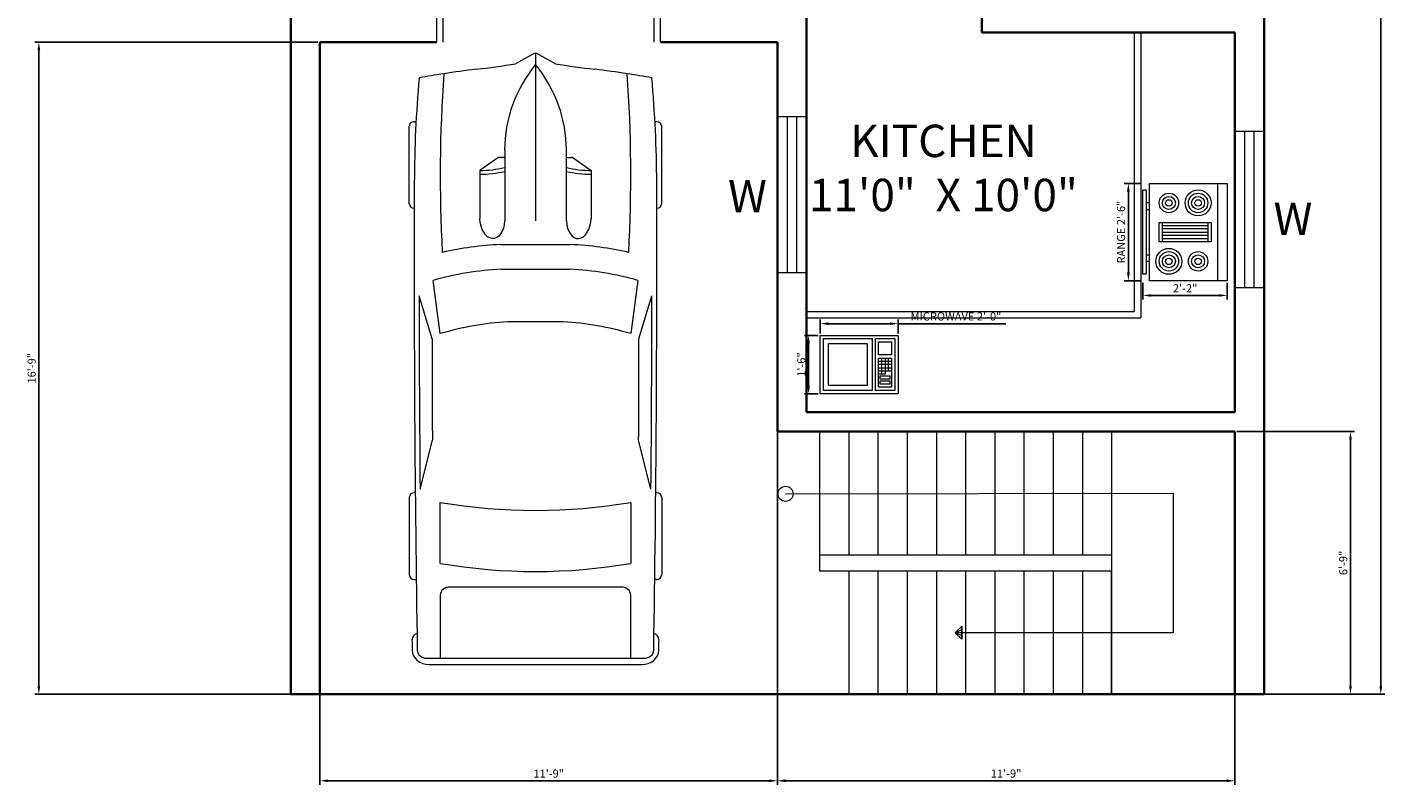
# Model space of a CAD drawing. Units: inches. Extents: x 2318 to 3542, y 1525 to 2117.
# Tile 1 of 6: x 2320 to 2739, y 1525 to 1758. Entities that reach past the tile are written whole.
import ezdxf

# ---------------------------------------------------------------- set-up
doc = ezdxf.new("R2010")
doc.units = ezdxf.units.IN
for name, color, linetype, lineweight in [('A-ANNO-DIMS', 2, 'Continuous', 18), ('A-ANNO-SYMB', 2, 'Continuous', 13), ('A-ANNO-TEXT', 7, 'Continuous', 18), ('A-AREA-IDEN', 7, 'Continuous', 25), ('A-DOOR', 4, 'Continuous', 18), ('A-EQPM', 9, 'Continuous', 18), ('A-FLOR-CASE', 8, 'Continuous', 18), ('A-FLOR-STRS', 3, 'Continuous', 18), ('A-GLAZ', 4, 'Continuous', 18), ('A-WALL', 7, 'Continuous', 35), ('C-PRKG', 8, 'Continuous', 13)]:
    doc.layers.add(name, color=color, linetype=linetype, lineweight=lineweight)
doc.styles.add('Annotative', font='arial.ttf')
doc.styles.get("Standard").update_dxf_attribs({"font": 'arial.ttf'})
doc.dimstyles.new('ISO-25', dxfattribs={"dimtxt": 2.5, "dimasz": 2.5, "dimexe": 1.25, "dimexo": 0.625, "dimtad": 1, "dimdec": 0, "dimlunit": 3, "dimtxsty": 'Standard', "dimcen": 2.5, "dimadec": 0, "dimazin": 0, "dimtfac": 1, "dimtdec": 0, "dimtmove": 0, "dimatfit": 3, "dimfxl": 1, "dimarcsym": 0})

# ---------------------------------------------------------------- blocks, each defined once
blk = doc.blocks.new('Range-Oven - 30 in top')
for p, q in [((0, -3), (30, -3)), ((12, -6), (18, -6)), ((13, -20), (13, -6)), ((14, -6), (14, -20)), ((15, -20), (15, -6)), ((16, -6), (16, -20)), ((17, -20), (17, -6)), ((18, -20), (12, -20)), ((6, -24), (6, -25)), ((8, -25), (8, -24)), ((22, -25), (22, -24)), ((24, -24), (24, -25))]:
    blk.add_line(p, q)
for points in [[(0, -24), (0, 0), (30, 0), (30, -24)], [(12, -21), (12, -5), (18, -5), (18, -21)], [(2, -26), (2, -25), (28, -25), (28, -26)]]:
    blk.add_lwpolyline(points, close=True)
for centre, radius in [((6, -9), 4), ((6, -9), 3), ((6, -9), 2), ((6, -9), 1), ((24, -9), 3), ((24, -9), 2), ((24, -9), 1), ((6, -18), 3), ((6, -18), 2), ((24, -18), 4), ((24, -18), 3), ((24, -18), 2), ((6, -18), 1), ((24, -18), 1)]:
    blk.add_circle(centre, radius)
blk = doc.blocks.new('Microwave')
for p, q in [((18, 10), (22, 10)), ((22, 9), (18, 9)), ((19, 7), (19, 11)), ((20, 11), (20, 7)), ((21, 7), (21, 11)), ((18, 8), (22, 8)), ((22, 7), (18, 7)), ((20, 6), (18, 6)), ((19, 6), (19, 7)), ((20, 7), (20, 6))]:
    blk.add_line(p, q)
for points in [[(0, 0), (0, 18), (24, 18), (24, 0)], [(1, 1), (1, 17), (16, 17), (16, 1)], [(17, 1), (17, 17), (23, 17), (23, 1)], [(2.5, 2.5), (2.5, 15.5), (14.5, 15.5), (14.5, 2.5)], [(18, 12), (18, 16), (22, 16), (22, 12)], [(18, 2), (18, 11), (22, 11), (22, 2)], [(18.5, 4.5), (18.5, 5.5), (21.5, 5.5), (21.5, 4.5)], [(18.5, 3), (18.5, 4), (21.5, 4), (21.5, 3)]]:
    blk.add_lwpolyline(points, close=True)
blk = doc.blocks.new('*U12')
for p, q in [((1182, 988), (568, 988)), ((3472, 988), (4087, 988)), ((536, 950), (536, 936)), ((1214, 950), (1214, 950)), ((2235, 810), (1899, 912)), ((3412, 904), (3030, 807)), ((3440, 942), (3440, 950)), ((4119, 950), (4119, 934)), ((4736, -851), (4736, 851)), ((1779, 801), (2195, 746)), ((3516, 746), (3994, 746)), ((4736, 746), (4242, 746)), ((4785, -832), (4785, 832)), ((4179, 670), (4179, -670)), ((820, 295), (918, 436)), ((918, 436), (1294, 436)), ((756, 241), (1313, 241)), ((816, 241), (816, 283)), ((1496, -274), (1496, 274)), ((1690, -267), (1690, 267)), ((2102, 216), (2102, -216)), ((4736, -267), (4736, 267)), ((83, 156), (3, 10)), ((0, 0), (1313, 0)), ((3, -10), (83, -156)), ((756, -241), (1313, -241)), ((816, -241), (816, -283)), ((820, -295), (918, -436)), ((918, -436), (1294, -436)), ((2195, -746), (1779, -801)), ((2235, -810), (1899, -912)), ((3412, -904), (3030, -807)), ((3994, -746), (3516, -746)), ((4242, -746), (4736, -746)), ((536, -950), (536, -936)), ((1214, -950), (1214, -950)), ((3440, -942), (3440, -950)), ((4119, -950), (4119, -934)), ((1182, -988), (568, -988)), ((3472, -988), (4087, -988))]:
    blk.add_line(p, q)
for centre, major_axis, ratio, start_param, end_param in [((568, 950), (0, -37.6), 0.842304, 3.141593, 4.712389), ((1182, 950), (0, 37.6), 0.842304, -1.570796, 0), ((3472, 950), (0, -37.6), 0.842304, 3.141593, 4.712389), ((4087, 950), (0, 37.6), 0.842304, -1.570796, 0), ((4588, 910), (0, 56.4), 0.842304, -0.013017, 1.249894), ((1638, -268131), (0, 269121), 0.842304, -0.013397, -0.013017), ((4673, 832), (0, -133), 0.842304, 1.570796, 3.128196), ((6757, -699), (0, 7958), 0.842304, 1.367076, 1.39176), ((1046, -12468), (0, 13417), 0.842304, 0.00281, 0.075598), ((1638, -268113), (0, 269063), 0.842304, -0.013397, 0.002797), ((1638, -268113), (0, -269025), 0.842304, 3.133765, 3.140441), ((4673, 851), (0, -75.2), 0.842304, 1.570796, 3.128196), ((952, -15087), (0, -15833), 0.842304, 3.096046, 3.200911), ((3436, 137), (0, 2077), 0.842304, 1.245306, 1.50788), ((3800, 71), (0, -2021), 0.842304, 4.372215, 4.640744), ((2433, -93125), (0, -93935), 0.842304, 3.134049, 3.144098), ((434, 0), (0, 3734), 0.842304, 4.511394, 4.913384), ((912, 0), (0, 3734), 0.842304, 4.511394, 4.913384), ((4242, 670), (0, 75.2), 0.842304, 0, 1.570796), ((6583, -699), (0, -7755), 0.842304, 4.528606, 4.561838), ((3414, 137), (0, -2280), 0.842304, 4.449482, 4.652344), ((-5194, 1331), (0, -6374), 0.842304, 1.385369, 1.434372), ((331, 432), (0, 696), 0.842304, 4.435146, 4.718221), ((361, 432), (0, 696), 0.842304, 4.435146, 4.718221), ((1290, 339), (161, -9), 0.603834, -1.395552, 1.581315), ((756, -1185), (0, 1427), 0.842304, 0, 0.590319), ((832, 283), (0, 18.8), 0.842304, 0.879714, 1.570796), ((16, 0), (0, -18.8), 0.842304, 4.131459, 5.293319), ((756, 1185), (0, 1427), 0.842304, 2.551274, 3.141593), ((-5194, -1331), (0, 6374), 0.842304, -1.434372, -1.385369), ((832, -283), (0, -18.8), 0.842304, 4.712389, 5.403472), ((331, -432), (0, -696), 0.842304, 1.564964, 1.848039), ((361, -432), (0, -696), 0.842304, 1.564964, 1.848039), ((3414, -137), (0, -2280), 0.842304, -1.510751, -1.307889), ((3436, -137), (0, -2077), 0.842304, -1.50788, -1.245306), ((3800, -71), (0, -2021), 0.842304, -1.499151, -1.230623), ((6583, 699), (0, 7755), 0.842304, 1.721348, 1.754579), ((6757, 699), (0, 7958), 0.842304, 1.749832, 1.774517), ((952, 15087), (0, -15833), 0.842304, -0.059319, 0.045547), ((4242, -670), (0, -75.2), 0.842304, 4.712389, 6.283185), ((2433, 93125), (0, -93935), 0.842304, -0.002505, 0.007544), ((4673, -832), (0, -133), 0.842304, 0.013397, 1.570796), ((1046, 12468), (0, -13417), 0.842304, -0.075598, -0.00281), ((568, -950), (0, 37.6), 0.842304, 1.570796, 3.141593), ((1638, 268113), (0, 269063), 0.842304, 3.138796, 3.15499), ((1182, -950), (0, -37.6), 0.842304, 0, 1.570796), ((1638, 268113), (0, -269025), 0.842304, 0.001152, 0.007828), ((3472, -950), (0, -37.6), 0.842304, -1.570796, 0), ((4087, -950), (0, 37.6), 0.842304, 3.141593, 4.712389), ((4588, -910), (0, -56.4), 0.842304, -1.249894, 0.013017), ((4673, -851), (0, 75.2), 0.842304, 3.15499, 4.712389), ((1638, 268131), (0, 269121), 0.842304, 3.15461, 3.15499)]:
    blk.add_ellipse(centre, major_axis=major_axis, ratio=ratio, start_param=start_param, end_param=end_param)
at = {"extrusion": (0, 0, -1)}
blk.add_ellipse((1290, -339), major_axis=(161, 9), ratio=0.603834, start_param=-1.395552, end_param=1.581315, dxfattribs=at)
blk = doc.blocks.new('*D16')
at = {"layer": 'A-ANNO-DIMS', "color": 0, "lineweight": -2, "transparency": 16777216}
for p, q in [((2702.28, 2032.62), (2738.91, 2032.62)), ((2737.66, 1555.12), (2737.66, 2030.12)), ((2702.28, 1552.62), (2738.91, 1552.62))]:
    blk.add_line(p, q, dxfattribs=at)
at = {"layer": 'A-ANNO-DIMS', "color": 0, "transparency": 16777216}
for points in [[(2737.24, 2030.12), (2738.07, 2030.12), (2737.66, 2032.62)], [(2737.24, 1555.12), (2738.07, 1555.12), (2737.66, 1552.62)]]:
    blk.add_solid(points, dxfattribs=at)
at = {"layer": 'Defpoints', "color": 0, "transparency": 16777216}
for p in [(2701.66, 2032.62), (2737.66, 2032.62), (2701.66, 1552.62)]:
    blk.add_point(p, dxfattribs=at)
at = {"layer": 'A-ANNO-DIMS', "color": 0, "transparency": 16777216, "insert": (2735.76, 1792.62), "char_height": 2.5, "attachment_point": 5, "rotation": 90}
blk.add_mtext("40'", dxfattribs=at)
blk = doc.blocks.new('WIN-48x9')
for p, q in [((48, 9), (0, 9)), ((0, 9), (0, 0)), ((48, 0), (48, 9)), ((48, 6), (0, 6)), ((0, 3), (48, 3)), ((0, 0), (48, 0))]:
    blk.add_line(p, q)
blk = doc.blocks.new('STAIR-ARROWHEAD')
for p, q in [((0, 2), (2, 4)), ((0, 2), (2, 3)), ((2, 2), (0, 2)), ((2, 0), (0, 2)), ((2, 1), (0, 2)), ((2, 2), (2, 4)), ((2, 4), (2, 2)), ((2, 4), (2, 0)), ((2, 3), (2, 1)), ((2, 2), (2, 0)), ((2, 0), (2, 2))]:
    blk.add_line(p, q)
blk = doc.blocks.new('*D46')
at = {"layer": 'A-ANNO-DIMS', "color": 0, "lineweight": -2, "transparency": 16777216}
for p, q in [((2663.72, 1710.07), (2658.59, 1710.07)), ((2659.84, 1707.57), (2659.84, 1682.57)), ((2663.72, 1680.07), (2658.59, 1680.07))]:
    blk.add_line(p, q, dxfattribs=at)
at = {"layer": 'A-ANNO-DIMS', "color": 0, "transparency": 16777216}
for points in [[(2659.42, 1707.57), (2660.26, 1707.57), (2659.84, 1710.07)], [(2659.42, 1682.57), (2660.26, 1682.57), (2659.84, 1680.07)]]:
    blk.add_solid(points, dxfattribs=at)
at = {"layer": 'Defpoints', "color": 0, "transparency": 16777216}
for p in [(2664.34, 1710.07), (2659.84, 1680.07), (2664.34, 1680.07)]:
    blk.add_point(p, dxfattribs=at)
at = {"layer": 'A-ANNO-DIMS', "color": 0, "transparency": 16777216, "insert": (2657.92, 1695.07), "char_height": 2.5, "attachment_point": 5, "rotation": 90}
blk.add_mtext('RANGE 2\'-6"', dxfattribs=at)
blk = doc.blocks.new('*D47')
at = {"layer": 'A-ANNO-DIMS', "color": 0, "lineweight": -2, "transparency": 16777216}
for p, q in [((2664.34, 1679.44), (2664.34, 1674.32)), ((2690.34, 1679.44), (2690.34, 1674.32)), ((2666.84, 1675.57), (2687.84, 1675.57))]:
    blk.add_line(p, q, dxfattribs=at)
at = {"layer": 'A-ANNO-DIMS', "color": 0, "transparency": 16777216}
for points in [[(2666.84, 1675.98), (2666.84, 1675.15), (2664.34, 1675.57)], [(2687.84, 1675.98), (2687.84, 1675.15), (2690.34, 1675.57)]]:
    blk.add_solid(points, dxfattribs=at)
at = {"layer": 'Defpoints', "color": 0, "transparency": 16777216}
for p in [(2664.34, 1680.07), (2690.34, 1680.07), (2690.34, 1675.57)]:
    blk.add_point(p, dxfattribs=at)
at = {"layer": 'A-ANNO-DIMS', "color": 0, "transparency": 16777216, "insert": (2677.34, 1677.45), "char_height": 2.5, "attachment_point": 5}
blk.add_mtext('2\'-2"', dxfattribs=at)
blk = doc.blocks.new('*D48')
at = {"layer": 'A-ANNO-DIMS', "color": 0, "lineweight": -2, "transparency": 16777216}
for p, q in [((2564.87, 1663.88), (2564.87, 1668.11)), ((2567.37, 1666.86), (2586.37, 1666.86)), ((2588.87, 1663.88), (2588.87, 1668.11)), ((2588.87, 1666.86), (2622.04, 1666.86))]:
    blk.add_line(p, q, dxfattribs=at)
at = {"layer": 'A-ANNO-DIMS', "color": 0, "transparency": 16777216}
for points in [[(2567.37, 1667.27), (2567.37, 1666.44), (2564.87, 1666.86)], [(2586.37, 1667.27), (2586.37, 1666.44), (2588.87, 1666.86)]]:
    blk.add_solid(points, dxfattribs=at)
at = {"layer": 'Defpoints', "color": 0, "transparency": 16777216}
for p in [(2588.87, 1666.86), (2564.87, 1663.26), (2588.87, 1663.26)]:
    blk.add_point(p, dxfattribs=at)
at = {"layer": 'A-ANNO-DIMS', "color": 0, "transparency": 16777216, "insert": (2606.7, 1668.77), "char_height": 2.5, "attachment_point": 5}
blk.add_mtext('MICROWAVE 2\'-0"', dxfattribs=at)
blk = doc.blocks.new('*D49')
at = {"layer": 'A-ANNO-DIMS', "color": 0, "lineweight": -2, "transparency": 16777216}
for p, q in [((2564.24, 1663.26), (2560.02, 1663.26)), ((2561.27, 1647.76), (2561.27, 1660.76)), ((2564.24, 1645.26), (2560.02, 1645.26))]:
    blk.add_line(p, q, dxfattribs=at)
at = {"layer": 'A-ANNO-DIMS', "color": 0, "transparency": 16777216}
for points in [[(2560.85, 1660.76), (2561.68, 1660.76), (2561.27, 1663.26)], [(2560.85, 1647.76), (2561.68, 1647.76), (2561.27, 1645.26)]]:
    blk.add_solid(points, dxfattribs=at)
at = {"layer": 'Defpoints', "color": 0, "transparency": 16777216}
for p in [(2561.27, 1663.26), (2564.87, 1663.26), (2564.87, 1645.26)]:
    blk.add_point(p, dxfattribs=at)
at = {"layer": 'A-ANNO-DIMS', "color": 0, "transparency": 16777216, "insert": (2559.36, 1654.26), "char_height": 2.5, "attachment_point": 5, "rotation": 90}
blk.add_mtext('1\'-6"', dxfattribs=at)
blk = doc.blocks.new('*D51')
at = {"layer": 'A-ANNO-DIMS', "color": 0, "lineweight": -2, "transparency": 16777216}
for p, q in [((2410.66, 1752.99), (2410.66, 1524.72)), ((2551.66, 1752.99), (2551.66, 1524.72)), ((2413.16, 1525.97), (2549.16, 1525.97))]:
    blk.add_line(p, q, dxfattribs=at)
at = {"layer": 'A-ANNO-DIMS', "color": 0, "transparency": 16777216}
for points in [[(2413.16, 1526.39), (2413.16, 1525.55), (2410.66, 1525.97)], [(2549.16, 1526.39), (2549.16, 1525.55), (2551.66, 1525.97)]]:
    blk.add_solid(points, dxfattribs=at)
at = {"layer": 'Defpoints', "color": 0, "transparency": 16777216}
for p in [(2410.66, 1753.62), (2551.66, 1753.62), (2551.66, 1525.97)]:
    blk.add_point(p, dxfattribs=at)
at = {"layer": 'A-ANNO-DIMS', "color": 0, "transparency": 16777216, "insert": (2481.16, 1527.87), "char_height": 2.5, "attachment_point": 5}
blk.add_mtext('11\'-9"', dxfattribs=at)
blk = doc.blocks.new('*D52')
at = {"layer": 'A-ANNO-DIMS', "color": 0, "lineweight": -2, "transparency": 16777216}
for p, q in [((2410.03, 1753.62), (2322.76, 1753.62)), ((2324.01, 1555.12), (2324.01, 1751.12)), ((2410.03, 1552.62), (2322.76, 1552.62))]:
    blk.add_line(p, q, dxfattribs=at)
at = {"layer": 'A-ANNO-DIMS', "color": 0, "transparency": 16777216}
for points in [[(2323.59, 1751.12), (2324.42, 1751.12), (2324.01, 1753.62)], [(2323.59, 1555.12), (2324.42, 1555.12), (2324.01, 1552.62)]]:
    blk.add_solid(points, dxfattribs=at)
at = {"layer": 'Defpoints', "color": 0, "transparency": 16777216}
for p in [(2324.01, 1753.62), (2410.66, 1753.62), (2410.66, 1552.62)]:
    blk.add_point(p, dxfattribs=at)
at = {"layer": 'A-ANNO-DIMS', "color": 0, "transparency": 16777216, "insert": (2322.11, 1653.12), "char_height": 2.5, "attachment_point": 5, "rotation": 90}
blk.add_mtext('16\'-9"', dxfattribs=at)
blk = doc.blocks.new('*D59')
at = {"layer": 'A-ANNO-DIMS', "color": 0, "lineweight": -2, "transparency": 16777216}
for p, q in [((2551.66, 1632.99), (2551.66, 1524.72)), ((2692.66, 1632.99), (2692.66, 1524.72)), ((2554.16, 1525.97), (2690.16, 1525.97))]:
    blk.add_line(p, q, dxfattribs=at)
at = {"layer": 'A-ANNO-DIMS', "color": 0, "transparency": 16777216}
for points in [[(2554.16, 1526.39), (2554.16, 1525.55), (2551.66, 1525.97)], [(2690.16, 1526.39), (2690.16, 1525.55), (2692.66, 1525.97)]]:
    blk.add_solid(points, dxfattribs=at)
at = {"layer": 'Defpoints', "color": 0, "transparency": 16777216}
for p in [(2551.66, 1633.62), (2692.66, 1633.62), (2692.66, 1525.97)]:
    blk.add_point(p, dxfattribs=at)
at = {"layer": 'A-ANNO-DIMS', "color": 0, "transparency": 16777216, "insert": (2622.16, 1527.87), "char_height": 2.5, "attachment_point": 5}
blk.add_mtext('11\'-9"', dxfattribs=at)
blk = doc.blocks.new('*D60')
at = {"layer": 'A-ANNO-DIMS', "color": 0, "lineweight": -2, "transparency": 16777216}
for p, q in [((2693.28, 1633.62), (2729.56, 1633.62)), ((2728.31, 1555.12), (2728.31, 1631.12)), ((2693.28, 1552.62), (2729.56, 1552.62))]:
    blk.add_line(p, q, dxfattribs=at)
at = {"layer": 'A-ANNO-DIMS', "color": 0, "transparency": 16777216}
for points in [[(2727.89, 1631.12), (2728.72, 1631.12), (2728.31, 1633.62)], [(2727.89, 1555.12), (2728.72, 1555.12), (2728.31, 1552.62)]]:
    blk.add_solid(points, dxfattribs=at)
at = {"layer": 'Defpoints', "color": 0, "transparency": 16777216}
for p in [(2692.66, 1633.62), (2728.31, 1633.62), (2692.66, 1552.62)]:
    blk.add_point(p, dxfattribs=at)
at = {"layer": 'A-ANNO-DIMS', "color": 0, "transparency": 16777216, "insert": (2726.41, 1593.12), "char_height": 2.5, "attachment_point": 5, "rotation": 90}
blk.add_mtext('6\'-9"', dxfattribs=at)

msp = doc.modelspace()

# ---------------------------------------------------------------- linework, layer by layer
at = {"layer": 'A-ANNO-SYMB'}
for p, q in [((2554.18, 1614.42), (2673.66, 1614.62)), ((2673.66, 1614.62), (2673.66, 1571.62)), ((2673.66, 1571.62), (2608.49, 1571.62))]:
    msp.add_line(p, q, dxfattribs=at)
msp.add_circle((2554.18, 1614.42), 2.33, dxfattribs=at)
at = {"layer": 'A-DOOR'}
for p, q in [((2446.66, 1753.62), (2446.66, 1762.62)), ((2448.66, 1753.62), (2448.66, 1762.62)), ((2513.66, 1753.62), (2513.66, 1762.62)), ((2515.66, 1753.62), (2515.66, 1762.62))]:
    msp.add_line(p, q, dxfattribs=at)
at = {"layer": 'A-FLOR-CASE'}
for p, q in [((2661.66, 1756.62), (2661.66, 1670.62)), ((2663.66, 1756.62), (2663.66, 1668.62)), ((2560.66, 1670.62), (2661.66, 1670.62)), ((2560.66, 1668.62), (2663.66, 1668.62))]:
    msp.add_line(p, q, dxfattribs=at)
at = {"layer": 'A-FLOR-STRS'}
for p, q in [((2564.66, 1633.62), (2564.66, 1590.62)), ((2573.66, 1633.62), (2573.66, 1595.62)), ((2582.66, 1633.62), (2582.66, 1595.62)), ((2591.66, 1633.62), (2591.66, 1595.62)), ((2600.66, 1633.62), (2600.66, 1595.62)), ((2609.66, 1633.62), (2609.66, 1595.62)), ((2618.66, 1633.62), (2618.66, 1595.62)), ((2627.66, 1633.62), (2627.66, 1595.62)), ((2636.66, 1633.62), (2636.66, 1595.62)), ((2645.66, 1633.62), (2645.66, 1595.62)), ((2654.66, 1633.62), (2654.66, 1595.62)), ((2564.66, 1595.62), (2654.66, 1595.62)), ((2654.66, 1595.62), (2654.66, 1590.62)), ((2654.66, 1590.62), (2564.66, 1590.62)), ((2573.66, 1590.62), (2573.66, 1552.62)), ((2582.66, 1590.62), (2582.66, 1552.62)), ((2591.66, 1590.62), (2591.66, 1552.62)), ((2600.66, 1590.62), (2600.66, 1552.62)), ((2609.66, 1590.62), (2609.66, 1552.62)), ((2618.66, 1590.62), (2618.66, 1552.62)), ((2627.66, 1590.62), (2627.66, 1552.62)), ((2636.66, 1590.62), (2636.66, 1552.62)), ((2645.66, 1590.62), (2645.66, 1552.62)), ((2654.66, 1590.62), (2654.66, 1552.62)), ((2654.66, 1552.62), (2654.66, 1590.62))]:
    msp.add_line(p, q, dxfattribs=at)
at = {"layer": 'A-WALL'}
for p, q in [((2401.66, 1552.62), (2401.66, 2032.62)), ((2701.66, 2032.62), (2701.66, 1552.62)), ((2560.66, 1756.62), (2560.66, 1762.62)), ((2614.66, 1762.62), (2614.66, 1756.62)), ((2410.66, 1552.62), (2410.66, 1753.62)), ((2410.66, 1753.62), (2446.66, 1753.62)), ((2410.66, 1753.62), (2446.66, 1753.62)), ((2551.66, 1753.62), (2515.66, 1753.62)), ((2515.66, 1753.62), (2551.66, 1753.62)), ((2551.66, 1753.62), (2551.66, 1639.62)), ((2551.66, 1753.62), (2551.66, 1753.62)), ((2560.66, 1756.62), (2560.66, 1639.62)), ((2614.66, 1756.62), (2692.66, 1756.62)), ((2692.66, 1756.62), (2692.66, 1639.62)), ((2551.66, 1639.62), (2551.66, 1633.62)), ((2560.66, 1639.62), (2692.66, 1639.62)), ((2554.66, 1633.62), (2551.66, 1633.62)), ((2554.66, 1633.62), (2692.66, 1633.62)), ((2692.66, 1633.62), (2654.66, 1633.62)), ((2692.66, 1633.62), (2692.66, 1552.62)), ((2701.66, 1552.62), (2401.66, 1552.62))]:
    msp.add_line(p, q, dxfattribs=at)

# ---------------------------------------------------------------- block references
at = {"layer": 'A-ANNO-SYMB'}
msp.add_blockref('STAIR-ARROWHEAD', (2606.49, 1569.62), dxfattribs=at)
at = {"layer": 'A-EQPM', "rotation": 270}
msp.add_blockref('Range-Oven - 30 in top', (2690.34, 1710.07), dxfattribs=at)
at = {"layer": 'A-EQPM'}
msp.add_blockref('Microwave', (2564.87, 1645.26), dxfattribs=at)
at = {"layer": 'A-GLAZ'}
for p, rotation in [((2560.66, 1682.59), 90.00000000000072), ((2701.66, 1678.06), 89.99999999999982)]:
    msp.add_blockref('WIN-48x9', p, dxfattribs=dict(at, rotation=rotation))
at = {"layer": 'C-PRKG', "xscale": 0.0393700787401575, "yscale": 0.0393700787401575, "zscale": 0.0393700787401575, "rotation": 270}
msp.add_blockref('*U12', (2477.1, 1750.21), dxfattribs=at)

# ---------------------------------------------------------------- texts
at = {"layer": 'A-ANNO-TEXT', "char_height": 10, "attachment_point": 1}
for insert in [(2536.44, 1711.14), (2704.6, 1704.17)]:
    msp.add_mtext_dynamic_manual_height_columns('\\pxt1;W', width=219.3474, gutter_width=12.5, heights=[0], dxfattribs=dict(at, insert=insert))
at = {"layer": 'A-AREA-IDEN', "insert": (2536.44, 1728.2), "char_height": 10, "width": 132.7792, "attachment_point": 1, "style": 'Annotative'}
msp.add_mtext('\\pxqc;KITCHEN\\P11\'0"  X 10\'0"', dxfattribs=at)

# ---------------------------------------------------------------- dimensions: what is measured, and where the dimension line sits
at = {"layer": 'A-ANNO-DIMS'}
for base, p1, p2, override, picture, middle in [((2737.66, 2032.62), (2701.66, 1552.62), (2701.66, 2032.62), {"dimclrd": 0, "dimclre": 0, "dimclrt": 0}, '*D16', (2735.76, 1792.62)), ((2324.01, 1753.62), (2410.66, 1552.62), (2410.66, 1753.62), {"dimdec": 1, "dimlfac": 1, "dimrnd": 0, "dimzin": 1, "dimdsep": 46, "dimlunit": 4, "dimfrac": 2}, '*D52', (2322.11, 1653.12)), ((2561.27, 1663.26), (2564.87, 1645.26), (2564.87, 1663.26), {"dimdec": 1, "dimlfac": 1, "dimrnd": 0, "dimzin": 1, "dimdsep": 46, "dimlunit": 4, "dimfrac": 2}, '*D49', (2559.36, 1654.26)), ((2728.31, 1633.62), (2692.66, 1552.62), (2692.66, 1633.62), {"dimdec": 1, "dimlfac": 1, "dimrnd": 0, "dimzin": 1, "dimdsep": 46, "dimlunit": 4, "dimfrac": 2}, '*D60', (2726.41, 1593.12))]:
    dim = msp.add_linear_dim(base=base, p1=p1, p2=p2, angle=90, dimstyle='ISO-25', override=override, dxfattribs=at)
    dim.commit()
    dim.dimension.update_dxf_attribs({"geometry": picture, "text_midpoint": middle})
for base, p1, p2, picture, middle in [((2551.66, 1525.97), (2410.66, 1753.62), (2551.66, 1753.62), '*D51', (2481.16, 1527.87)), ((2690.34, 1675.57), (2664.34, 1680.07), (2690.34, 1680.07), '*D47', (2677.34, 1677.45)), ((2692.66, 1525.97), (2551.66, 1633.62), (2692.66, 1633.62), '*D59', (2622.16, 1527.87))]:
    dim = msp.add_linear_dim(base=base, p1=p1, p2=p2, dimstyle='ISO-25', override={"dimdec": 1, "dimlfac": 1, "dimrnd": 0, "dimzin": 1, "dimdsep": 46, "dimlunit": 4, "dimfrac": 2}, dxfattribs=at)
    dim.commit()
    dim.dimension.update_dxf_attribs({"geometry": picture, "text_midpoint": middle})
dim = msp.add_linear_dim(base=(2659.84, 1680.07), p1=(2664.34, 1710.07), p2=(2664.34, 1680.07), angle=270, text='RANGE <>', dimstyle='ISO-25', override={"dimdec": 1, "dimlfac": 1, "dimrnd": 0, "dimzin": 1, "dimdsep": 46, "dimlunit": 4, "dimfrac": 2}, dxfattribs=at)
dim.commit()
dim.dimension.update_dxf_attribs({"geometry": '*D46', "text_midpoint": (2657.92, 1695.07)})
dim = msp.add_linear_dim(base=(2588.87, 1666.86), p1=(2564.87, 1663.26), p2=(2588.87, 1663.26), text='MICROWAVE <>', dimstyle='ISO-25', override={"dimdec": 1, "dimlfac": 1, "dimrnd": 0, "dimzin": 1, "dimdsep": 46, "dimlunit": 4, "dimfrac": 2}, dxfattribs=at)
dim.commit()
dim.dimension.update_dxf_attribs({"geometry": '*D48', "text_midpoint": (2606.7, 1668.77)})

doc.saveas('drawing.dxf')
